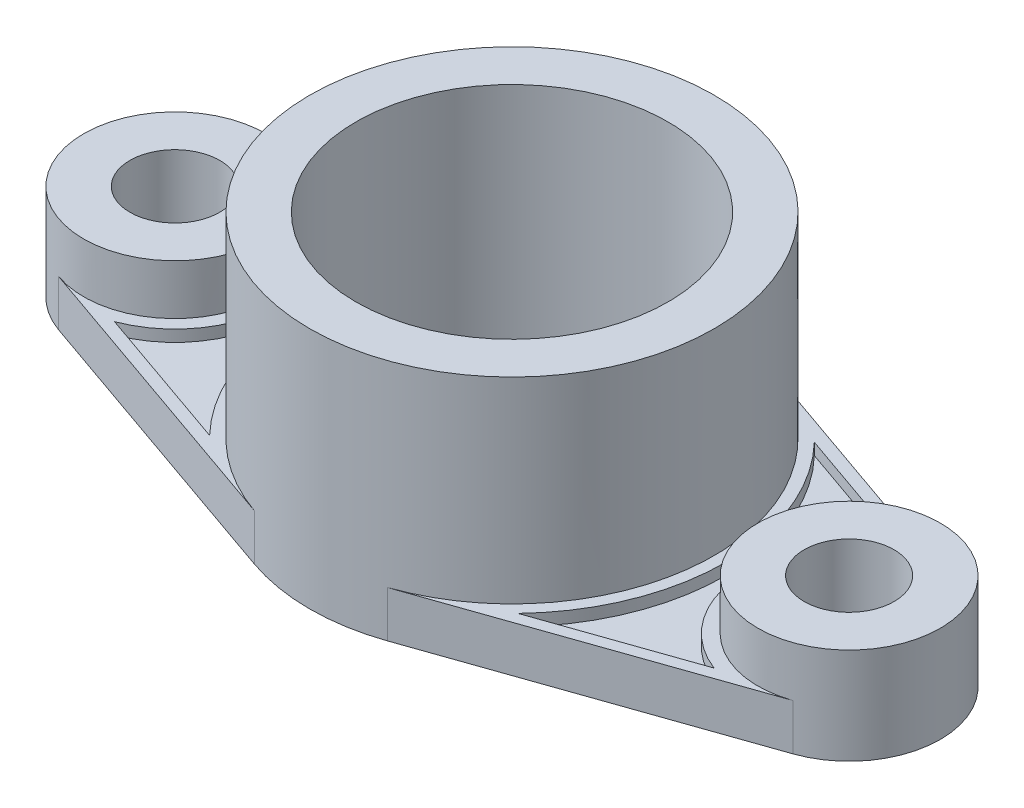
ISO-10303-21;
HEADER;
FILE_DESCRIPTION(('STEP AP214'),'2;1');
FILE_NAME('part.step','',(''),(''),'','','');
FILE_SCHEMA(('AUTOMOTIVE_DESIGN { 1 0 10303 214 1 1 1 1 }'));
ENDSEC;
DATA;
#1=APPLICATION_CONTEXT('core data for automotive mechanical design processes');
#2=APPLICATION_PROTOCOL_DEFINITION('international standard','automotive_design',2000,#1);
#3=PRODUCT_CONTEXT('',#1,'mechanical');
#4=PRODUCT('Part','Part','',(#3));
#5=PRODUCT_RELATED_PRODUCT_CATEGORY('part','',(#4));
#6=PRODUCT_DEFINITION_FORMATION('','',#4);
#7=PRODUCT_DEFINITION_CONTEXT('part definition',#1,'design');
#8=PRODUCT_DEFINITION('design','',#6,#7);
#9=PRODUCT_DEFINITION_SHAPE('','',#8);
#10=(LENGTH_UNIT() NAMED_UNIT(*) SI_UNIT(.MILLI.,.METRE.));
#11=(NAMED_UNIT(*) PLANE_ANGLE_UNIT() SI_UNIT($,.RADIAN.));
#12=(NAMED_UNIT(*) SI_UNIT($,.STERADIAN.) SOLID_ANGLE_UNIT());
#13=UNCERTAINTY_MEASURE_WITH_UNIT(LENGTH_MEASURE(1.E-05),#10,'distance_accuracy_value','');
#14=(GEOMETRIC_REPRESENTATION_CONTEXT(3) GLOBAL_UNCERTAINTY_ASSIGNED_CONTEXT((#13)) GLOBAL_UNIT_ASSIGNED_CONTEXT((#10,
#11,#12)) REPRESENTATION_CONTEXT('',''));
#15=CARTESIAN_POINT('',(0.,0.,0.));
#16=DIRECTION('',(0.,0.,1.));
#17=DIRECTION('',(1.,0.,0.));
#18=AXIS2_PLACEMENT_3D('',#15,#16,#17);
#19=CARTESIAN_POINT('',(0.,63.,0.));
#20=DIRECTION('',(0.,-1.,0.));
#21=DIRECTION('',(0.,0.,-1.));
#22=AXIS2_PLACEMENT_3D('',#19,#20,#21);
#23=CYLINDRICAL_SURFACE('',#22,40.5);
#24=CARTESIAN_POINT('',(0.,63.,0.));
#25=DIRECTION('',(0.,1.,0.));
#26=DIRECTION('',(0.,0.,1.));
#27=AXIS2_PLACEMENT_3D('',#24,#25,#26);
#28=CIRCLE('',#27,40.5);
#29=CARTESIAN_POINT('',(0.,63.,40.5));
#30=VERTEX_POINT('',#29);
#31=EDGE_CURVE('E47',#30,#30,#28,.T.);
#32=ORIENTED_EDGE('',*,*,#31,.T.);
#33=EDGE_LOOP('',(#32));
#34=FACE_BOUND('',#33,.T.);
#35=CARTESIAN_POINT('',(0.,0.,0.));
#36=DIRECTION('',(0.,1.,0.));
#37=DIRECTION('',(0.,0.,1.));
#38=AXIS2_PLACEMENT_3D('',#35,#36,#37);
#39=CIRCLE('',#38,40.5);
#40=CARTESIAN_POINT('',(0.,0.,40.5));
#41=VERTEX_POINT('',#40);
#42=EDGE_CURVE('E277',#41,#41,#39,.T.);
#43=ORIENTED_EDGE('',*,*,#42,.F.);
#44=EDGE_LOOP('',(#43));
#45=FACE_BOUND('',#44,.T.);
#46=ADVANCED_FACE('F41',(#34,#45),#23,.F.);
#47=CARTESIAN_POINT('',(0.,63.,0.));
#48=DIRECTION('',(0.,-1.,0.));
#49=DIRECTION('',(0.,0.,-1.));
#50=AXIS2_PLACEMENT_3D('',#47,#48,#49);
#51=CYLINDRICAL_SURFACE('',#50,52.5);
#52=CARTESIAN_POINT('',(0.,12.,0.));
#53=DIRECTION('',(0.,1.,0.));
#54=DIRECTION('',(0.,0.,1.));
#55=AXIS2_PLACEMENT_3D('',#52,#53,#54);
#56=CIRCLE('',#55,52.5);
#57=CARTESIAN_POINT('',(-17.300000001,12.,-49.5677314385619));
#58=VERTEX_POINT('',#57);
#59=CARTESIAN_POINT('',(-17.300000001,12.,49.5677314385619));
#60=VERTEX_POINT('',#59);
#61=EDGE_CURVE('E254',#58,#60,#56,.T.);
#62=ORIENTED_EDGE('',*,*,#61,.T.);
#63=DIRECTION('',(0.,-1.,0.));
#64=VECTOR('',#63,1.);
#65=CARTESIAN_POINT('',(-17.300000001,12.,49.5677314385619));
#66=LINE('',#65,#64);
#67=CARTESIAN_POINT('',(-17.300000001,0.,49.5677314385619));
#68=VERTEX_POINT('',#67);
#69=EDGE_CURVE('E271',#60,#68,#66,.T.);
#70=ORIENTED_EDGE('',*,*,#69,.T.);
#71=CARTESIAN_POINT('',(0.,0.,0.));
#72=DIRECTION('',(0.,1.,0.));
#73=DIRECTION('',(0.,0.,1.));
#74=AXIS2_PLACEMENT_3D('',#71,#72,#73);
#75=CIRCLE('',#74,52.5);
#76=CARTESIAN_POINT('',(17.300000001,0.,49.5677314385619));
#77=VERTEX_POINT('',#76);
#78=EDGE_CURVE('E42',#68,#77,#75,.T.);
#79=ORIENTED_EDGE('',*,*,#78,.T.);
#80=DIRECTION('',(0.,-1.,0.));
#81=VECTOR('',#80,1.);
#82=CARTESIAN_POINT('',(17.300000001,12.,49.5677314385619));
#83=LINE('',#82,#81);
#84=CARTESIAN_POINT('',(17.300000001,12.,49.5677314385619));
#85=VERTEX_POINT('',#84);
#86=EDGE_CURVE('E293',#85,#77,#83,.T.);
#87=ORIENTED_EDGE('',*,*,#86,.F.);
#88=CARTESIAN_POINT('',(0.,12.,0.));
#89=DIRECTION('',(0.,1.,0.));
#90=DIRECTION('',(0.,0.,1.));
#91=AXIS2_PLACEMENT_3D('',#88,#89,#90);
#92=CIRCLE('',#91,52.5);
#93=CARTESIAN_POINT('',(17.300000001,12.,-49.5677314385619));
#94=VERTEX_POINT('',#93);
#95=EDGE_CURVE('E284',#85,#94,#92,.T.);
#96=ORIENTED_EDGE('',*,*,#95,.T.);
#97=DIRECTION('',(0.,-1.,0.));
#98=VECTOR('',#97,1.);
#99=CARTESIAN_POINT('',(17.300000001,12.,-49.5677314385619));
#100=LINE('',#99,#98);
#101=CARTESIAN_POINT('',(17.300000001,0.,-49.5677314385619));
#102=VERTEX_POINT('',#101);
#103=EDGE_CURVE('E296',#94,#102,#100,.T.);
#104=ORIENTED_EDGE('',*,*,#103,.T.);
#105=CARTESIAN_POINT('',(-17.300000001,0.,-49.5677314385619));
#106=VERTEX_POINT('',#105);
#107=EDGE_CURVE('E305',#102,#106,#75,.T.);
#108=ORIENTED_EDGE('',*,*,#107,.T.);
#109=DIRECTION('',(0.,-1.,0.));
#110=VECTOR('',#109,1.);
#111=CARTESIAN_POINT('',(-17.300000001,12.,-49.5677314385619));
#112=LINE('',#111,#110);
#113=EDGE_CURVE('E268',#58,#106,#112,.T.);
#114=ORIENTED_EDGE('',*,*,#113,.F.);
#115=EDGE_LOOP('',(#62,#70,#79,#87,#96,#104,#108,#114));
#116=FACE_BOUND('',#115,.T.);
#117=CARTESIAN_POINT('',(0.,63.,0.));
#118=DIRECTION('',(0.,1.,0.));
#119=DIRECTION('',(0.,0.,1.));
#120=AXIS2_PLACEMENT_3D('',#117,#118,#119);
#121=CIRCLE('',#120,52.5);
#122=CARTESIAN_POINT('',(0.,63.,52.5));
#123=VERTEX_POINT('',#122);
#124=EDGE_CURVE('E11',#123,#123,#121,.T.);
#125=ORIENTED_EDGE('',*,*,#124,.F.);
#126=EDGE_LOOP('',(#125));
#127=FACE_BOUND('',#126,.T.);
#128=ADVANCED_FACE('F306',(#116,#127),#51,.T.);
#129=CARTESIAN_POINT('',(0.,63.,0.));
#130=DIRECTION('',(0.,1.,0.));
#131=DIRECTION('',(0.,0.,1.));
#132=AXIS2_PLACEMENT_3D('',#129,#130,#131);
#133=PLANE('',#132);
#134=ORIENTED_EDGE('',*,*,#31,.F.);
#135=EDGE_LOOP('',(#134));
#136=FACE_BOUND('',#135,.T.);
#137=ORIENTED_EDGE('',*,*,#124,.T.);
#138=EDGE_LOOP('',(#137));
#139=FACE_BOUND('',#138,.T.);
#140=ADVANCED_FACE('F349',(#136,#139),#133,.T.);
#141=CARTESIAN_POINT('',(0.,0.,0.));
#142=DIRECTION('',(0.,1.,0.));
#143=DIRECTION('',(0.,0.,1.));
#144=AXIS2_PLACEMENT_3D('',#141,#142,#143);
#145=PLANE('',#144);
#146=ORIENTED_EDGE('',*,*,#42,.T.);
#147=EDGE_LOOP('',(#146));
#148=FACE_BOUND('',#147,.T.);
#149=ORIENTED_EDGE('',*,*,#107,.F.);
#150=DIRECTION('',(0.944147265496418,0.,0.329523809542857));
#151=VECTOR('',#150,1.);
#152=CARTESIAN_POINT('',(17.300000001,0.,-49.5677314385619));
#153=LINE('',#152,#151);
#154=CARTESIAN_POINT('',(95.2987301586317,0.,-22.344818615175));
#155=VERTEX_POINT('',#154);
#156=EDGE_CURVE('E234',#102,#155,#153,.T.);
#157=ORIENTED_EDGE('',*,*,#156,.T.);
#158=CARTESIAN_POINT('',(87.5,0.,0.));
#159=DIRECTION('',(0.,1.,0.));
#160=DIRECTION('',(0.,0.,1.));
#161=AXIS2_PLACEMENT_3D('',#158,#159,#160);
#162=CIRCLE('',#161,23.666666665);
#163=CARTESIAN_POINT('',(95.2987301586317,0.,22.344818615175));
#164=VERTEX_POINT('',#163);
#165=EDGE_CURVE('E243',#164,#155,#162,.T.);
#166=ORIENTED_EDGE('',*,*,#165,.F.);
#167=DIRECTION('',(0.944147265496418,0.,-0.329523809542857));
#168=VECTOR('',#167,1.);
#169=CARTESIAN_POINT('',(17.300000001,0.,49.5677314385619));
#170=LINE('',#169,#168);
#171=EDGE_CURVE('E283',#77,#164,#170,.T.);
#172=ORIENTED_EDGE('',*,*,#171,.F.);
#173=ORIENTED_EDGE('',*,*,#78,.F.);
#174=DIRECTION('',(-0.944147265496418,0.,-0.329523809542857));
#175=VECTOR('',#174,1.);
#176=CARTESIAN_POINT('',(-17.300000001,0.,49.5677314385619));
#177=LINE('',#176,#175);
#178=CARTESIAN_POINT('',(-95.2987301586317,0.,22.344818615175));
#179=VERTEX_POINT('',#178);
#180=EDGE_CURVE('E261',#68,#179,#177,.T.);
#181=ORIENTED_EDGE('',*,*,#180,.T.);
#182=CARTESIAN_POINT('',(-87.5,0.,0.));
#183=DIRECTION('',(0.,1.,0.));
#184=DIRECTION('',(0.,0.,1.));
#185=AXIS2_PLACEMENT_3D('',#182,#183,#184);
#186=CIRCLE('',#185,23.666666665);
#187=CARTESIAN_POINT('',(-95.2987301586317,0.,-22.344818615175));
#188=VERTEX_POINT('',#187);
#189=EDGE_CURVE('E226',#188,#179,#186,.T.);
#190=ORIENTED_EDGE('',*,*,#189,.F.);
#191=DIRECTION('',(-0.944147265496418,0.,0.329523809542857));
#192=VECTOR('',#191,1.);
#193=CARTESIAN_POINT('',(-17.300000001,0.,-49.5677314385619));
#194=LINE('',#193,#192);
#195=EDGE_CURVE('E252',#106,#188,#194,.T.);
#196=ORIENTED_EDGE('',*,*,#195,.F.);
#197=EDGE_LOOP('',(#149,#157,#166,#172,#173,#181,#190,#196));
#198=FACE_BOUND('',#197,.T.);
#199=CARTESIAN_POINT('',(-87.5,0.,0.));
#200=DIRECTION('',(0.,1.,0.));
#201=DIRECTION('',(0.,0.,1.));
#202=AXIS2_PLACEMENT_3D('',#199,#200,#201);
#203=CIRCLE('',#202,11.666666665);
#204=CARTESIAN_POINT('',(-87.5,0.,11.666666665));
#205=VERTEX_POINT('',#204);
#206=EDGE_CURVE('E231',#205,#205,#203,.T.);
#207=ORIENTED_EDGE('',*,*,#206,.T.);
#208=EDGE_LOOP('',(#207));
#209=FACE_BOUND('',#208,.T.);
#210=CARTESIAN_POINT('',(87.5,0.,0.));
#211=DIRECTION('',(0.,1.,0.));
#212=DIRECTION('',(0.,0.,1.));
#213=AXIS2_PLACEMENT_3D('',#210,#211,#212);
#214=CIRCLE('',#213,11.666666665);
#215=CARTESIAN_POINT('',(87.5,0.,11.666666665));
#216=VERTEX_POINT('',#215);
#217=EDGE_CURVE('E187',#216,#216,#214,.T.);
#218=ORIENTED_EDGE('',*,*,#217,.T.);
#219=EDGE_LOOP('',(#218));
#220=FACE_BOUND('',#219,.T.);
#221=ADVANCED_FACE('F317',(#148,#198,#209,#220),#145,.F.);
#222=CARTESIAN_POINT('',(17.300000001,12.,-49.5677314385619));
#223=DIRECTION('',(0.329523809542857,0.,-0.944147265496418));
#224=DIRECTION('',(-0.944147265496418,0.,-0.329523809542857));
#225=AXIS2_PLACEMENT_3D('',#222,#223,#224);
#226=PLANE('',#225);
#227=ORIENTED_EDGE('',*,*,#156,.F.);
#228=ORIENTED_EDGE('',*,*,#103,.F.);
#229=DIRECTION('',(0.944147265496418,0.,0.329523809542857));
#230=VECTOR('',#229,1.);
#231=CARTESIAN_POINT('',(17.300000001,12.,-49.5677314385619));
#232=LINE('',#231,#230);
#233=CARTESIAN_POINT('',(95.2987301586317,12.,-22.344818615175));
#234=VERTEX_POINT('',#233);
#235=EDGE_CURVE('E278',#94,#234,#232,.T.);
#236=ORIENTED_EDGE('',*,*,#235,.T.);
#237=DIRECTION('',(0.,-1.,0.));
#238=VECTOR('',#237,1.);
#239=CARTESIAN_POINT('',(95.2987301586317,12.,-22.344818615175));
#240=LINE('',#239,#238);
#241=EDGE_CURVE('E262',#234,#155,#240,.T.);
#242=ORIENTED_EDGE('',*,*,#241,.T.);
#243=EDGE_LOOP('',(#227,#228,#236,#242));
#244=FACE_BOUND('',#243,.T.);
#245=ADVANCED_FACE('F358',(#244),#226,.T.);
#246=CARTESIAN_POINT('',(17.300000001,12.,49.5677314385619));
#247=DIRECTION('',(-0.329523809542857,0.,-0.944147265496418));
#248=DIRECTION('',(-0.944147265496418,0.,0.329523809542857));
#249=AXIS2_PLACEMENT_3D('',#246,#247,#248);
#250=PLANE('',#249);
#251=ORIENTED_EDGE('',*,*,#171,.T.);
#252=DIRECTION('',(0.,-1.,0.));
#253=VECTOR('',#252,1.);
#254=CARTESIAN_POINT('',(95.2987301586317,12.,22.344818615175));
#255=LINE('',#254,#253);
#256=CARTESIAN_POINT('',(95.2987301586317,12.,22.344818615175));
#257=VERTEX_POINT('',#256);
#258=EDGE_CURVE('E288',#257,#164,#255,.T.);
#259=ORIENTED_EDGE('',*,*,#258,.F.);
#260=DIRECTION('',(0.944147265496418,0.,-0.329523809542857));
#261=VECTOR('',#260,1.);
#262=CARTESIAN_POINT('',(17.300000001,12.,49.5677314385619));
#263=LINE('',#262,#261);
#264=EDGE_CURVE('E289',#85,#257,#263,.T.);
#265=ORIENTED_EDGE('',*,*,#264,.F.);
#266=ORIENTED_EDGE('',*,*,#86,.T.);
#267=EDGE_LOOP('',(#251,#259,#265,#266));
#268=FACE_BOUND('',#267,.T.);
#269=ADVANCED_FACE('F337',(#268),#250,.F.);
#270=CARTESIAN_POINT('',(0.,12.,0.));
#271=DIRECTION('',(0.,1.,0.));
#272=DIRECTION('',(0.,0.,1.));
#273=AXIS2_PLACEMENT_3D('',#270,#271,#272);
#274=PLANE('',#273);
#275=CARTESIAN_POINT('',(87.5,12.,0.));
#276=DIRECTION('',(0.,-1.,0.));
#277=DIRECTION('',(0.,0.,1.));
#278=AXIS2_PLACEMENT_3D('',#275,#276,#277);
#279=CIRCLE('',#278,27.1182125827807);
#280=CARTESIAN_POINT('',(77.7327409572556,12.,25.2981838177528));
#281=VERTEX_POINT('',#280);
#282=CARTESIAN_POINT('',(77.7327409572556,12.,-25.2981838177528));
#283=VERTEX_POINT('',#282);
#284=EDGE_CURVE('E60',#281,#283,#279,.T.);
#285=ORIENTED_EDGE('',*,*,#284,.F.);
#286=DIRECTION('',(0.944147265496418,0.,-0.329523809542857));
#287=VECTOR('',#286,1.);
#288=CARTESIAN_POINT('',(40.0093368584407,12.,38.4643076650006));
#289=LINE('',#288,#287);
#290=CARTESIAN_POINT('',(40.0093368584407,12.,38.4643076650006));
#291=VERTEX_POINT('',#290);
#292=EDGE_CURVE('E172',#291,#281,#289,.T.);
#293=ORIENTED_EDGE('',*,*,#292,.F.);
#294=CARTESIAN_POINT('',(0.,12.,0.));
#295=DIRECTION('',(0.,-1.,0.));
#296=DIRECTION('',(0.,0.,1.));
#297=AXIS2_PLACEMENT_3D('',#294,#295,#296);
#298=CIRCLE('',#297,55.5);
#299=CARTESIAN_POINT('',(40.0093368584407,12.,-38.4643076650005));
#300=VERTEX_POINT('',#299);
#301=EDGE_CURVE('E180',#300,#291,#298,.T.);
#302=ORIENTED_EDGE('',*,*,#301,.F.);
#303=DIRECTION('',(-0.944147265496418,0.,-0.329523809542857));
#304=VECTOR('',#303,1.);
#305=CARTESIAN_POINT('',(40.0093368584407,12.,-38.4643076650005));
#306=LINE('',#305,#304);
#307=EDGE_CURVE('E184',#283,#300,#306,.T.);
#308=ORIENTED_EDGE('',*,*,#307,.F.);
#309=EDGE_LOOP('',(#285,#293,#302,#308));
#310=FACE_BOUND('',#309,.T.);
#311=CARTESIAN_POINT('',(87.5,12.,0.));
#312=DIRECTION('',(0.,1.,0.));
#313=DIRECTION('',(0.,0.,1.));
#314=AXIS2_PLACEMENT_3D('',#311,#312,#313);
#315=CIRCLE('',#314,23.666666665);
#316=EDGE_CURVE('E280',#234,#257,#315,.T.);
#317=ORIENTED_EDGE('',*,*,#316,.F.);
#318=ORIENTED_EDGE('',*,*,#235,.F.);
#319=ORIENTED_EDGE('',*,*,#95,.F.);
#320=ORIENTED_EDGE('',*,*,#264,.T.);
#321=EDGE_LOOP('',(#317,#318,#319,#320));
#322=FACE_BOUND('',#321,.T.);
#323=ADVANCED_FACE('F335',(#310,#322),#274,.T.);
#324=CARTESIAN_POINT('',(-17.300000001,12.,49.5677314385619));
#325=DIRECTION('',(-0.329523809542857,0.,0.944147265496418));
#326=DIRECTION('',(0.944147265496418,0.,0.329523809542857));
#327=AXIS2_PLACEMENT_3D('',#324,#325,#326);
#328=PLANE('',#327);
#329=ORIENTED_EDGE('',*,*,#180,.F.);
#330=ORIENTED_EDGE('',*,*,#69,.F.);
#331=DIRECTION('',(-0.944147265496418,0.,-0.329523809542857));
#332=VECTOR('',#331,1.);
#333=CARTESIAN_POINT('',(-17.300000001,12.,49.5677314385619));
#334=LINE('',#333,#332);
#335=CARTESIAN_POINT('',(-95.2987301586317,12.,22.344818615175));
#336=VERTEX_POINT('',#335);
#337=EDGE_CURVE('E253',#60,#336,#334,.T.);
#338=ORIENTED_EDGE('',*,*,#337,.T.);
#339=DIRECTION('',(0.,-1.,0.));
#340=VECTOR('',#339,1.);
#341=CARTESIAN_POINT('',(-95.2987301586317,12.,22.344818615175));
#342=LINE('',#341,#340);
#343=EDGE_CURVE('E273',#336,#179,#342,.T.);
#344=ORIENTED_EDGE('',*,*,#343,.T.);
#345=EDGE_LOOP('',(#329,#330,#338,#344));
#346=FACE_BOUND('',#345,.T.);
#347=ADVANCED_FACE('F329',(#346),#328,.T.);
#348=CARTESIAN_POINT('',(-17.300000001,12.,-49.5677314385619));
#349=DIRECTION('',(0.329523809542857,0.,0.944147265496418));
#350=DIRECTION('',(0.944147265496418,0.,-0.329523809542857));
#351=AXIS2_PLACEMENT_3D('',#348,#349,#350);
#352=PLANE('',#351);
#353=ORIENTED_EDGE('',*,*,#195,.T.);
#354=DIRECTION('',(0.,-1.,0.));
#355=VECTOR('',#354,1.);
#356=CARTESIAN_POINT('',(-95.2987301586317,12.,-22.344818615175));
#357=LINE('',#356,#355);
#358=CARTESIAN_POINT('',(-95.2987301586317,12.,-22.344818615175));
#359=VERTEX_POINT('',#358);
#360=EDGE_CURVE('E257',#359,#188,#357,.T.);
#361=ORIENTED_EDGE('',*,*,#360,.F.);
#362=DIRECTION('',(-0.944147265496418,0.,0.329523809542857));
#363=VECTOR('',#362,1.);
#364=CARTESIAN_POINT('',(-17.300000001,12.,-49.5677314385619));
#365=LINE('',#364,#363);
#366=EDGE_CURVE('E260',#58,#359,#365,.T.);
#367=ORIENTED_EDGE('',*,*,#366,.F.);
#368=ORIENTED_EDGE('',*,*,#113,.T.);
#369=EDGE_LOOP('',(#353,#361,#367,#368));
#370=FACE_BOUND('',#369,.T.);
#371=ADVANCED_FACE('F316',(#370),#352,.F.);
#372=CARTESIAN_POINT('',(0.,12.,0.));
#373=DIRECTION('',(0.,1.,0.));
#374=DIRECTION('',(0.,0.,1.));
#375=AXIS2_PLACEMENT_3D('',#372,#373,#374);
#376=PLANE('',#375);
#377=CARTESIAN_POINT('',(-87.5,12.,0.));
#378=DIRECTION('',(0.,-1.,0.));
#379=DIRECTION('',(0.,0.,1.));
#380=AXIS2_PLACEMENT_3D('',#377,#378,#379);
#381=CIRCLE('',#380,27.0050609760334);
#382=CARTESIAN_POINT('',(-77.8982228402785,12.,-25.2404277636956));
#383=VERTEX_POINT('',#382);
#384=CARTESIAN_POINT('',(-77.8982228402785,12.,25.2404277636956));
#385=VERTEX_POINT('',#384);
#386=EDGE_CURVE('E62',#383,#385,#381,.T.);
#387=ORIENTED_EDGE('',*,*,#386,.F.);
#388=DIRECTION('',(-0.944147265496417,0.,0.329523809542857));
#389=VECTOR('',#388,1.);
#390=CARTESIAN_POINT('',(-40.0093368584407,12.,-38.4643076650006));
#391=LINE('',#390,#389);
#392=CARTESIAN_POINT('',(-40.0093368584407,12.,-38.4643076650006));
#393=VERTEX_POINT('',#392);
#394=EDGE_CURVE('E201',#393,#383,#391,.T.);
#395=ORIENTED_EDGE('',*,*,#394,.F.);
#396=CARTESIAN_POINT('',(0.,12.,0.));
#397=DIRECTION('',(0.,-1.,0.));
#398=DIRECTION('',(0.,0.,1.));
#399=AXIS2_PLACEMENT_3D('',#396,#397,#398);
#400=CIRCLE('',#399,55.5);
#401=CARTESIAN_POINT('',(-40.0093368584407,12.,38.4643076650005));
#402=VERTEX_POINT('',#401);
#403=EDGE_CURVE('E206',#402,#393,#400,.T.);
#404=ORIENTED_EDGE('',*,*,#403,.F.);
#405=DIRECTION('',(0.944147265496418,0.,0.329523809542857));
#406=VECTOR('',#405,1.);
#407=CARTESIAN_POINT('',(-40.0093368584407,12.,38.4643076650005));
#408=LINE('',#407,#406);
#409=EDGE_CURVE('E209',#385,#402,#408,.T.);
#410=ORIENTED_EDGE('',*,*,#409,.F.);
#411=EDGE_LOOP('',(#387,#395,#404,#410));
#412=FACE_BOUND('',#411,.T.);
#413=CARTESIAN_POINT('',(-87.5,12.,0.));
#414=DIRECTION('',(0.,1.,0.));
#415=DIRECTION('',(0.,0.,1.));
#416=AXIS2_PLACEMENT_3D('',#413,#414,#415);
#417=CIRCLE('',#416,23.666666665);
#418=EDGE_CURVE('E250',#336,#359,#417,.T.);
#419=ORIENTED_EDGE('',*,*,#418,.F.);
#420=ORIENTED_EDGE('',*,*,#337,.F.);
#421=ORIENTED_EDGE('',*,*,#61,.F.);
#422=ORIENTED_EDGE('',*,*,#366,.T.);
#423=EDGE_LOOP('',(#419,#420,#421,#422));
#424=FACE_BOUND('',#423,.T.);
#425=ADVANCED_FACE('F326',(#412,#424),#376,.T.);
#426=CARTESIAN_POINT('',(-87.5,25.,0.));
#427=DIRECTION('',(0.,-1.,0.));
#428=DIRECTION('',(0.,0.,-1.));
#429=AXIS2_PLACEMENT_3D('',#426,#427,#428);
#430=CYLINDRICAL_SURFACE('',#429,23.666666665);
#431=CARTESIAN_POINT('',(-87.5,25.,0.));
#432=DIRECTION('',(0.,1.,0.));
#433=DIRECTION('',(0.,0.,1.));
#434=AXIS2_PLACEMENT_3D('',#431,#432,#433);
#435=CIRCLE('',#434,23.666666665);
#436=CARTESIAN_POINT('',(-87.5,25.,23.666666665));
#437=VERTEX_POINT('',#436);
#438=EDGE_CURVE('E230',#437,#437,#435,.T.);
#439=ORIENTED_EDGE('',*,*,#438,.F.);
#440=EDGE_LOOP('',(#439));
#441=FACE_BOUND('',#440,.T.);
#442=ORIENTED_EDGE('',*,*,#189,.T.);
#443=ORIENTED_EDGE('',*,*,#343,.F.);
#444=ORIENTED_EDGE('',*,*,#418,.T.);
#445=ORIENTED_EDGE('',*,*,#360,.T.);
#446=EDGE_LOOP('',(#442,#443,#444,#445));
#447=FACE_BOUND('',#446,.T.);
#448=ADVANCED_FACE('F322',(#441,#447),#430,.T.);
#449=CARTESIAN_POINT('',(-87.5,25.,0.));
#450=DIRECTION('',(0.,-1.,0.));
#451=DIRECTION('',(0.,0.,-1.));
#452=AXIS2_PLACEMENT_3D('',#449,#450,#451);
#453=CYLINDRICAL_SURFACE('',#452,11.666666665);
#454=CARTESIAN_POINT('',(-87.5,25.,0.));
#455=DIRECTION('',(0.,1.,0.));
#456=DIRECTION('',(0.,0.,1.));
#457=AXIS2_PLACEMENT_3D('',#454,#455,#456);
#458=CIRCLE('',#457,11.666666665);
#459=CARTESIAN_POINT('',(-87.5,25.,11.666666665));
#460=VERTEX_POINT('',#459);
#461=EDGE_CURVE('E221',#460,#460,#458,.T.);
#462=ORIENTED_EDGE('',*,*,#461,.T.);
#463=EDGE_LOOP('',(#462));
#464=FACE_BOUND('',#463,.T.);
#465=ORIENTED_EDGE('',*,*,#206,.F.);
#466=EDGE_LOOP('',(#465));
#467=FACE_BOUND('',#466,.T.);
#468=ADVANCED_FACE('F386',(#464,#467),#453,.F.);
#469=CARTESIAN_POINT('',(0.,25.,0.));
#470=DIRECTION('',(0.,1.,0.));
#471=DIRECTION('',(0.,0.,1.));
#472=AXIS2_PLACEMENT_3D('',#469,#470,#471);
#473=PLANE('',#472);
#474=ORIENTED_EDGE('',*,*,#461,.F.);
#475=EDGE_LOOP('',(#474));
#476=FACE_BOUND('',#475,.T.);
#477=ORIENTED_EDGE('',*,*,#438,.T.);
#478=EDGE_LOOP('',(#477));
#479=FACE_BOUND('',#478,.T.);
#480=ADVANCED_FACE('F377',(#476,#479),#473,.T.);
#481=CARTESIAN_POINT('',(87.5,25.,0.));
#482=DIRECTION('',(0.,-1.,0.));
#483=DIRECTION('',(0.,0.,-1.));
#484=AXIS2_PLACEMENT_3D('',#481,#482,#483);
#485=CYLINDRICAL_SURFACE('',#484,23.666666665);
#486=CARTESIAN_POINT('',(87.5,25.,0.));
#487=DIRECTION('',(0.,1.,0.));
#488=DIRECTION('',(0.,0.,1.));
#489=AXIS2_PLACEMENT_3D('',#486,#487,#488);
#490=CIRCLE('',#489,23.666666665);
#491=CARTESIAN_POINT('',(87.5,25.,23.666666665));
#492=VERTEX_POINT('',#491);
#493=EDGE_CURVE('E232',#492,#492,#490,.T.);
#494=ORIENTED_EDGE('',*,*,#493,.F.);
#495=EDGE_LOOP('',(#494));
#496=FACE_BOUND('',#495,.T.);
#497=ORIENTED_EDGE('',*,*,#165,.T.);
#498=ORIENTED_EDGE('',*,*,#241,.F.);
#499=ORIENTED_EDGE('',*,*,#316,.T.);
#500=ORIENTED_EDGE('',*,*,#258,.T.);
#501=EDGE_LOOP('',(#497,#498,#499,#500));
#502=FACE_BOUND('',#501,.T.);
#503=ADVANCED_FACE('F375',(#496,#502),#485,.T.);
#504=CARTESIAN_POINT('',(87.5,25.,0.));
#505=DIRECTION('',(0.,-1.,0.));
#506=DIRECTION('',(0.,0.,-1.));
#507=AXIS2_PLACEMENT_3D('',#504,#505,#506);
#508=CYLINDRICAL_SURFACE('',#507,11.666666665);
#509=CARTESIAN_POINT('',(87.5,25.,0.));
#510=DIRECTION('',(0.,1.,0.));
#511=DIRECTION('',(0.,0.,1.));
#512=AXIS2_PLACEMENT_3D('',#509,#510,#511);
#513=CIRCLE('',#512,11.666666665);
#514=CARTESIAN_POINT('',(87.5,25.,11.666666665));
#515=VERTEX_POINT('',#514);
#516=EDGE_CURVE('E236',#515,#515,#513,.T.);
#517=ORIENTED_EDGE('',*,*,#516,.T.);
#518=EDGE_LOOP('',(#517));
#519=FACE_BOUND('',#518,.T.);
#520=ORIENTED_EDGE('',*,*,#217,.F.);
#521=EDGE_LOOP('',(#520));
#522=FACE_BOUND('',#521,.T.);
#523=ADVANCED_FACE('F378',(#519,#522),#508,.F.);
#524=CARTESIAN_POINT('',(0.,25.,0.));
#525=DIRECTION('',(0.,1.,0.));
#526=DIRECTION('',(0.,0.,1.));
#527=AXIS2_PLACEMENT_3D('',#524,#525,#526);
#528=PLANE('',#527);
#529=ORIENTED_EDGE('',*,*,#516,.F.);
#530=EDGE_LOOP('',(#529));
#531=FACE_BOUND('',#530,.T.);
#532=ORIENTED_EDGE('',*,*,#493,.T.);
#533=EDGE_LOOP('',(#532));
#534=FACE_BOUND('',#533,.T.);
#535=ADVANCED_FACE('F387',(#531,#534),#528,.T.);
#536=CARTESIAN_POINT('',(-87.5,9.,0.));
#537=DIRECTION('',(0.,1.,0.));
#538=DIRECTION('',(0.,0.,1.));
#539=AXIS2_PLACEMENT_3D('',#536,#537,#538);
#540=CYLINDRICAL_SURFACE('',#539,27.0050609760334);
#541=ORIENTED_EDGE('',*,*,#386,.T.);
#542=DIRECTION('',(0.,1.,0.));
#543=VECTOR('',#542,1.);
#544=CARTESIAN_POINT('',(-77.8982228402785,9.,25.2404277636956));
#545=LINE('',#544,#543);
#546=CARTESIAN_POINT('',(-77.8982228402785,9.,25.2404277636956));
#547=VERTEX_POINT('',#546);
#548=EDGE_CURVE('E193',#547,#385,#545,.T.);
#549=ORIENTED_EDGE('',*,*,#548,.F.);
#550=CARTESIAN_POINT('',(-87.5,9.,0.));
#551=DIRECTION('',(0.,-1.,0.));
#552=DIRECTION('',(0.,0.,1.));
#553=AXIS2_PLACEMENT_3D('',#550,#551,#552);
#554=CIRCLE('',#553,27.0050609760334);
#555=CARTESIAN_POINT('',(-77.8982228402785,9.,-25.2404277636956));
#556=VERTEX_POINT('',#555);
#557=EDGE_CURVE('E210',#556,#547,#554,.T.);
#558=ORIENTED_EDGE('',*,*,#557,.F.);
#559=DIRECTION('',(0.,1.,0.));
#560=VECTOR('',#559,1.);
#561=CARTESIAN_POINT('',(-77.8982228402785,9.,-25.2404277636956));
#562=LINE('',#561,#560);
#563=EDGE_CURVE('E203',#556,#383,#562,.T.);
#564=ORIENTED_EDGE('',*,*,#563,.T.);
#565=EDGE_LOOP('',(#541,#549,#558,#564));
#566=FACE_BOUND('',#565,.T.);
#567=ADVANCED_FACE('F411',(#566),#540,.T.);
#568=CARTESIAN_POINT('',(-40.0093368584407,9.,-38.4643076650006));
#569=DIRECTION('',(-0.329523809542857,0.,-0.944147265496418));
#570=DIRECTION('',(-0.944147265496418,0.,0.329523809542857));
#571=AXIS2_PLACEMENT_3D('',#568,#569,#570);
#572=PLANE('',#571);
#573=ORIENTED_EDGE('',*,*,#394,.T.);
#574=ORIENTED_EDGE('',*,*,#563,.F.);
#575=DIRECTION('',(-0.944147265496417,0.,0.329523809542857));
#576=VECTOR('',#575,1.);
#577=CARTESIAN_POINT('',(-40.0093368584407,9.,-38.4643076650006));
#578=LINE('',#577,#576);
#579=CARTESIAN_POINT('',(-40.0093368584407,9.,-38.4643076650006));
#580=VERTEX_POINT('',#579);
#581=EDGE_CURVE('E198',#580,#556,#578,.T.);
#582=ORIENTED_EDGE('',*,*,#581,.F.);
#583=DIRECTION('',(0.,1.,0.));
#584=VECTOR('',#583,1.);
#585=CARTESIAN_POINT('',(-40.0093368584407,9.,-38.4643076650006));
#586=LINE('',#585,#584);
#587=EDGE_CURVE('E200',#580,#393,#586,.T.);
#588=ORIENTED_EDGE('',*,*,#587,.T.);
#589=EDGE_LOOP('',(#573,#574,#582,#588));
#590=FACE_BOUND('',#589,.T.);
#591=ADVANCED_FACE('F417',(#590),#572,.F.);
#592=CARTESIAN_POINT('',(0.,9.,0.));
#593=DIRECTION('',(0.,1.,0.));
#594=DIRECTION('',(0.,0.,1.));
#595=AXIS2_PLACEMENT_3D('',#592,#593,#594);
#596=CYLINDRICAL_SURFACE('',#595,55.5);
#597=ORIENTED_EDGE('',*,*,#403,.T.);
#598=ORIENTED_EDGE('',*,*,#587,.F.);
#599=CARTESIAN_POINT('',(0.,9.,0.));
#600=DIRECTION('',(0.,-1.,0.));
#601=DIRECTION('',(0.,0.,1.));
#602=AXIS2_PLACEMENT_3D('',#599,#600,#601);
#603=CIRCLE('',#602,55.5);
#604=CARTESIAN_POINT('',(-40.0093368584407,9.,38.4643076650005));
#605=VERTEX_POINT('',#604);
#606=EDGE_CURVE('E216',#605,#580,#603,.T.);
#607=ORIENTED_EDGE('',*,*,#606,.F.);
#608=DIRECTION('',(0.,1.,0.));
#609=VECTOR('',#608,1.);
#610=CARTESIAN_POINT('',(-40.0093368584407,9.,38.4643076650005));
#611=LINE('',#610,#609);
#612=EDGE_CURVE('E197',#605,#402,#611,.T.);
#613=ORIENTED_EDGE('',*,*,#612,.T.);
#614=EDGE_LOOP('',(#597,#598,#607,#613));
#615=FACE_BOUND('',#614,.T.);
#616=ADVANCED_FACE('F420',(#615),#596,.T.);
#617=CARTESIAN_POINT('',(-40.0093368584407,9.,38.4643076650005));
#618=DIRECTION('',(-0.329523809542857,0.,0.944147265496417));
#619=DIRECTION('',(0.944147265496418,0.,0.329523809542857));
#620=AXIS2_PLACEMENT_3D('',#617,#618,#619);
#621=PLANE('',#620);
#622=ORIENTED_EDGE('',*,*,#409,.T.);
#623=ORIENTED_EDGE('',*,*,#612,.F.);
#624=DIRECTION('',(0.944147265496418,0.,0.329523809542857));
#625=VECTOR('',#624,1.);
#626=CARTESIAN_POINT('',(-40.0093368584407,9.,38.4643076650005));
#627=LINE('',#626,#625);
#628=EDGE_CURVE('E218',#547,#605,#627,.T.);
#629=ORIENTED_EDGE('',*,*,#628,.F.);
#630=ORIENTED_EDGE('',*,*,#548,.T.);
#631=EDGE_LOOP('',(#622,#623,#629,#630));
#632=FACE_BOUND('',#631,.T.);
#633=ADVANCED_FACE('F406',(#632),#621,.F.);
#634=CARTESIAN_POINT('',(-87.5,9.,0.));
#635=DIRECTION('',(0.,1.,0.));
#636=DIRECTION('',(0.,0.,1.));
#637=AXIS2_PLACEMENT_3D('',#634,#635,#636);
#638=PLANE('',#637);
#639=ORIENTED_EDGE('',*,*,#557,.T.);
#640=ORIENTED_EDGE('',*,*,#628,.T.);
#641=ORIENTED_EDGE('',*,*,#606,.T.);
#642=ORIENTED_EDGE('',*,*,#581,.T.);
#643=EDGE_LOOP('',(#639,#640,#641,#642));
#644=FACE_BOUND('',#643,.T.);
#645=ADVANCED_FACE('F412',(#644),#638,.T.);
#646=CARTESIAN_POINT('',(87.5,9.,0.));
#647=DIRECTION('',(0.,1.,0.));
#648=DIRECTION('',(0.,0.,1.));
#649=AXIS2_PLACEMENT_3D('',#646,#647,#648);
#650=CYLINDRICAL_SURFACE('',#649,27.1182125827807);
#651=ORIENTED_EDGE('',*,*,#284,.T.);
#652=DIRECTION('',(0.,1.,0.));
#653=VECTOR('',#652,1.);
#654=CARTESIAN_POINT('',(77.7327409572556,9.,-25.2981838177528));
#655=LINE('',#654,#653);
#656=CARTESIAN_POINT('',(77.7327409572556,9.,-25.2981838177528));
#657=VERTEX_POINT('',#656);
#658=EDGE_CURVE('E153',#657,#283,#655,.T.);
#659=ORIENTED_EDGE('',*,*,#658,.F.);
#660=CARTESIAN_POINT('',(87.5,9.,0.));
#661=DIRECTION('',(0.,-1.,0.));
#662=DIRECTION('',(0.,0.,1.));
#663=AXIS2_PLACEMENT_3D('',#660,#661,#662);
#664=CIRCLE('',#663,27.1182125827807);
#665=CARTESIAN_POINT('',(77.7327409572556,9.,25.2981838177528));
#666=VERTEX_POINT('',#665);
#667=EDGE_CURVE('E160',#666,#657,#664,.T.);
#668=ORIENTED_EDGE('',*,*,#667,.F.);
#669=DIRECTION('',(0.,1.,0.));
#670=VECTOR('',#669,1.);
#671=CARTESIAN_POINT('',(77.7327409572556,9.,25.2981838177528));
#672=LINE('',#671,#670);
#673=EDGE_CURVE('E186',#666,#281,#672,.T.);
#674=ORIENTED_EDGE('',*,*,#673,.T.);
#675=EDGE_LOOP('',(#651,#659,#668,#674));
#676=FACE_BOUND('',#675,.T.);
#677=ADVANCED_FACE('F154',(#676),#650,.T.);
#678=CARTESIAN_POINT('',(40.0093368584407,9.,38.4643076650006));
#679=DIRECTION('',(0.329523809542857,0.,0.944147265496417));
#680=DIRECTION('',(0.944147265496418,0.,-0.329523809542857));
#681=AXIS2_PLACEMENT_3D('',#678,#679,#680);
#682=PLANE('',#681);
#683=ORIENTED_EDGE('',*,*,#292,.T.);
#684=ORIENTED_EDGE('',*,*,#673,.F.);
#685=DIRECTION('',(0.944147265496418,0.,-0.329523809542857));
#686=VECTOR('',#685,1.);
#687=CARTESIAN_POINT('',(40.0093368584407,9.,38.4643076650006));
#688=LINE('',#687,#686);
#689=CARTESIAN_POINT('',(40.0093368584407,9.,38.4643076650006));
#690=VERTEX_POINT('',#689);
#691=EDGE_CURVE('E162',#690,#666,#688,.T.);
#692=ORIENTED_EDGE('',*,*,#691,.F.);
#693=DIRECTION('',(0.,1.,0.));
#694=VECTOR('',#693,1.);
#695=CARTESIAN_POINT('',(40.0093368584407,9.,38.4643076650006));
#696=LINE('',#695,#694);
#697=EDGE_CURVE('E194',#690,#291,#696,.T.);
#698=ORIENTED_EDGE('',*,*,#697,.T.);
#699=EDGE_LOOP('',(#683,#684,#692,#698));
#700=FACE_BOUND('',#699,.T.);
#701=ADVANCED_FACE('F509',(#700),#682,.F.);
#702=CARTESIAN_POINT('',(0.,9.,0.));
#703=DIRECTION('',(0.,1.,0.));
#704=DIRECTION('',(0.,0.,1.));
#705=AXIS2_PLACEMENT_3D('',#702,#703,#704);
#706=CYLINDRICAL_SURFACE('',#705,55.5);
#707=ORIENTED_EDGE('',*,*,#301,.T.);
#708=ORIENTED_EDGE('',*,*,#697,.F.);
#709=CARTESIAN_POINT('',(0.,9.,0.));
#710=DIRECTION('',(0.,-1.,0.));
#711=DIRECTION('',(0.,0.,1.));
#712=AXIS2_PLACEMENT_3D('',#709,#710,#711);
#713=CIRCLE('',#712,55.5);
#714=CARTESIAN_POINT('',(40.0093368584407,9.,-38.4643076650005));
#715=VERTEX_POINT('',#714);
#716=EDGE_CURVE('E173',#715,#690,#713,.T.);
#717=ORIENTED_EDGE('',*,*,#716,.F.);
#718=DIRECTION('',(0.,1.,0.));
#719=VECTOR('',#718,1.);
#720=CARTESIAN_POINT('',(40.0093368584407,9.,-38.4643076650005));
#721=LINE('',#720,#719);
#722=EDGE_CURVE('E165',#715,#300,#721,.T.);
#723=ORIENTED_EDGE('',*,*,#722,.T.);
#724=EDGE_LOOP('',(#707,#708,#717,#723));
#725=FACE_BOUND('',#724,.T.);
#726=ADVANCED_FACE('F513',(#725),#706,.T.);
#727=CARTESIAN_POINT('',(40.0093368584407,9.,-38.4643076650005));
#728=DIRECTION('',(0.329523809542857,0.,-0.944147265496418));
#729=DIRECTION('',(-0.944147265496418,0.,-0.329523809542857));
#730=AXIS2_PLACEMENT_3D('',#727,#728,#729);
#731=PLANE('',#730);
#732=ORIENTED_EDGE('',*,*,#307,.T.);
#733=ORIENTED_EDGE('',*,*,#722,.F.);
#734=DIRECTION('',(-0.944147265496418,0.,-0.329523809542857));
#735=VECTOR('',#734,1.);
#736=CARTESIAN_POINT('',(40.0093368584407,9.,-38.4643076650005));
#737=LINE('',#736,#735);
#738=EDGE_CURVE('E167',#657,#715,#737,.T.);
#739=ORIENTED_EDGE('',*,*,#738,.F.);
#740=ORIENTED_EDGE('',*,*,#658,.T.);
#741=EDGE_LOOP('',(#732,#733,#739,#740));
#742=FACE_BOUND('',#741,.T.);
#743=ADVANCED_FACE('F170',(#742),#731,.F.);
#744=CARTESIAN_POINT('',(87.5,9.,0.));
#745=DIRECTION('',(0.,1.,0.));
#746=DIRECTION('',(0.,0.,1.));
#747=AXIS2_PLACEMENT_3D('',#744,#745,#746);
#748=PLANE('',#747);
#749=ORIENTED_EDGE('',*,*,#667,.T.);
#750=ORIENTED_EDGE('',*,*,#738,.T.);
#751=ORIENTED_EDGE('',*,*,#716,.T.);
#752=ORIENTED_EDGE('',*,*,#691,.T.);
#753=EDGE_LOOP('',(#749,#750,#751,#752));
#754=FACE_BOUND('',#753,.T.);
#755=ADVANCED_FACE('F171',(#754),#748,.T.);
#756=CLOSED_SHELL('',(#46,#128,#140,#221,#245,#269,#323,#347,#371,#425,#448,#468,#480,#503,#523,
#535,#567,#591,#616,#633,#645,#677,#701,#726,#743,#755));
#757=MANIFOLD_SOLID_BREP('B2',#756);
#758=ADVANCED_BREP_SHAPE_REPRESENTATION('',(#18,#757),#14);
#759=SHAPE_DEFINITION_REPRESENTATION(#9,#758);
ENDSEC;
END-ISO-10303-21;
